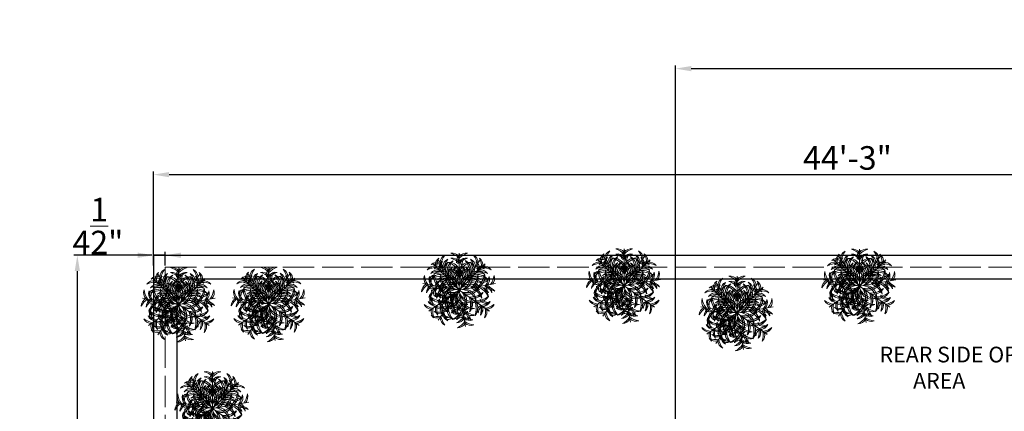
# Model space of a CAD drawing. Units: millimetres. Extents: x 595116 to 630915, y 909473 to 920225.
# Tile 124 of 134: x 629260 to 629637, y 920030 to 920179. Entities that reach past the tile are written whole.
import ezdxf

# ---------------------------------------------------------------- set-up
doc = ezdxf.new("R2010")
doc.units = ezdxf.units.MM
doc.linetypes.add('ACAD_ISO02W100', pattern=[15, 12, -3])
for name, color, linetype, lineweight in [('A-AREA-IDEN', 7, 'Continuous', 20), ('C-PROP', 7, 'Continuous', 25), ('C-PROP-REF', 240, 'ACAD_ISO02W100', 13), ('Dimension', 3, 'Continuous', 18), ('L-PLNT', 85, 'Continuous', 13)]:
    doc.layers.add(name, color=color, linetype=linetype, lineweight=lineweight)
doc.styles.get("Standard").update_dxf_attribs({"font": 'arial.ttf'})
doc.dimstyles.new('ISO-25', dxfattribs={"dimtxt": 9, "dimasz": 6, "dimexe": 1.25, "dimexo": 0.625, "dimtad": 1, "dimlunit": 4, "dimtxsty": 'Standard', "dimcen": 2.5, "dimadec": 0, "dimazin": 0, "dimtfac": 1, "dimtmove": 0, "dimatfit": 3, "dimfxl": 1, "dimarcsym": 0})

# ---------------------------------------------------------------- blocks, each defined once
blk = doc.blocks.new('A$C5D061C3B')
for p, q in [((3.377, 6.679), (3.377, 3.377)), ((1.03, 5.716), (3.365, 3.381)), ((1.483, 6.082), (3.377, 3.377)), ((5.259, 6.086), (3.365, 3.381)), ((5.712, 5.712), (3.377, 3.377)), ((0.125, 3.951), (3.377, 3.377)), ((6.629, 3.951), (3.377, 3.377)), ((0.66, 1.487), (3.365, 3.381)), ((1.483, 0.672), (3.377, 3.377)), ((6.07, 1.487), (3.365, 3.381)), ((3.951, 0.125), (3.377, 3.377)), ((6.082, 1.483), (3.377, 3.377))]:
    blk.add_line(p, q)
for centre, radius, start, end in [((1.998, 5.617), 0.762, 125.37567, 188.71003), ((3.066, 5.423), 1.715, 151.62064, 180.92372), ((2.419, 5.816), 0.762, 115.37567, 178.71003), ((3.438, 5.44), 1.715, 141.62064, 170.92372), ((2.763, 5.924), 0.762, 36.28997, 99.62433), ((2.145, 5.032), 1.715, 44.07628, 73.37936), ((2.763, 5.474), 0.762, 36.28997, 99.62433), ((2.145, 4.581), 1.715, 44.07628, 73.37936), ((3.901, 5.939), 0.762, 125.37567, 188.71003), ((4.969, 5.745), 1.715, 151.62064, 180.92372), ((3.991, 5.924), 0.762, 80.37567, 143.71003), ((4.61, 5.032), 1.715, 106.62064, 135.92372), ((3.991, 5.474), 0.762, 80.37567, 143.71003), ((4.61, 4.581), 1.715, 106.62064, 135.92372), ((3.871, 5.832), 0.38, 94.742, 213.74753), ((4.447, 5.681), 0.826, 139.61802, 183.21064), ((3.305, 5.444), 1.715, 9.07628, 38.37936), ((4.323, 5.82), 0.762, 1.28997, 64.62433), ((4.744, 5.613), 0.762, 351.28997, 54.62433), ((3.676, 5.419), 1.715, 359.07628, 28.37936), ((1.13, 4.748), 0.762, 81.28997, 144.62433), ((1.324, 3.68), 1.715, 89.07628, 118.37936), ((1.413, 5.111), 0.762, 71.28997, 134.62433), ((1.419, 4.026), 1.715, 79.07628, 108.37936), ((1.671, 4.742), 0.762, 71.28997, 134.62433), ((1.677, 3.657), 1.715, 79.07628, 108.37936), ((2.317, 5.298), 0.762, 125.37567, 188.71003), ((1.991, 5.462), 0.38, 139.742, 258.74753), ((3.385, 5.104), 1.715, 151.62064, 180.92372), ((2.505, 5.763), 0.826, 184.61802, 228.21064), ((2.678, 5.447), 0.762, 115.37567, 178.71003), ((3.035, 5.062), 1.056, 129.60629, 199.75109), ((3.696, 5.07), 1.715, 141.62064, 170.92372), ((3.894, 4.989), 1.77, 149.96343, 193.62881), ((3.344, 5.089), 1.056, 119.60629, 189.75109), ((2.422, 4.799), 1.056, 25.24891, 95.39371), ((1.866, 4.14), 1.77, 31.37119, 75.03657), ((3.46, 4.637), 1.056, 129.60629, 199.75109), ((4.177, 4.869), 1.77, 139.96343, 183.62881), ((4.319, 4.565), 1.77, 149.96343, 193.62881), ((3.688, 4.597), 1.056, 119.60629, 189.75109), ((4.522, 4.377), 1.77, 139.96343, 183.62881), ((4.332, 4.799), 1.056, 84.60629, 154.75109), ((4.888, 4.14), 1.77, 104.96343, 148.62881), ((2.221, 4.381), 1.77, 356.37119, 40.03657), ((3.054, 4.602), 1.056, 350.24891, 60.39371), ((3.398, 5.094), 1.056, 350.24891, 60.39371), ((2.565, 4.873), 1.77, 356.37119, 40.03657), ((3.283, 4.633), 1.056, 340.24891, 50.39371), ((2.424, 4.56), 1.77, 346.37119, 30.03657), ((2.848, 4.985), 1.77, 346.37119, 30.03657), ((3.707, 5.058), 1.056, 340.24891, 50.39371), ((4.064, 5.451), 0.762, 1.28997, 64.62433), ((3.046, 5.075), 1.715, 9.07628, 38.37936), ((5.065, 3.661), 1.715, 71.62064, 100.92372), ((5.071, 4.746), 0.762, 45.37567, 108.71003), ((3.357, 5.1), 1.715, 359.07628, 28.37936), ((4.425, 5.294), 0.762, 351.28997, 54.62433), ((5.564, 4.807), 0.762, 80.37567, 143.71003), ((6.182, 3.914), 1.715, 106.62064, 135.92372), ((5.419, 3.676), 1.715, 61.62064, 90.92372), ((5.613, 4.744), 0.762, 35.37567, 98.71003), ((0.975, 4.424), 0.762, 160.37567, 223.71003), ((1.962, 4.878), 1.715, 186.62064, 215.92372), ((1.419, 4.346), 0.762, 160.37567, 223.71003), ((2.405, 4.8), 1.715, 186.62064, 215.92372), ((1.12, 4.31), 0.38, 94.742, 213.74753), ((1.448, 4.43), 0.762, 81.28997, 144.62433), ((1.642, 3.362), 1.715, 89.07628, 118.37936), ((1.696, 4.159), 0.826, 139.61802, 183.21064), ((1.685, 3.712), 1.056, 70.24891, 140.39371), ((1.757, 2.853), 1.77, 76.37119, 120.03657), ((2.143, 4.564), 1.056, 164.60629, 234.75109), ((1.78, 3.994), 1.056, 60.24891, 130.39371), ((1.702, 3.136), 1.77, 66.37119, 110.03657), ((2.888, 4.998), 1.77, 184.96343, 228.62881), ((2.124, 3.502), 1.056, 60.24891, 130.39371), ((2.046, 2.644), 1.77, 66.37119, 110.03657), ((2.734, 4.46), 1.056, 164.60629, 234.75109), ((3.48, 4.893), 1.77, 184.96343, 228.62881), ((2.358, 3.686), 1.029, 3.42594, 103.63458), ((1.93, 3.14), 1.557, 21.66646, 83.18779), ((3.25, 4.435), 1.029, 156.36542, 256.57406), ((3.862, 4.761), 1.557, 176.81221, 238.33354), ((2.422, 4.198), 1.056, 25.24891, 95.39371), ((1.866, 3.54), 1.77, 31.37119, 75.03657), ((3.868, 4.321), 1.029, 121.36542, 221.57406), ((4.556, 4.237), 1.557, 141.81221, 203.33354), ((4.035, 4.215), 1.029, 111.36542, 211.57406), ((2.707, 4.219), 1.029, 328.42594, 68.63458), ((2.044, 4.017), 1.557, 346.66646, 48.18779), ((4.698, 4.013), 1.557, 131.81221, 193.33354), ((4.397, 3.686), 1.029, 76.36542, 176.57406), ((4.332, 4.198), 1.056, 84.60629, 154.75109), ((4.888, 3.54), 1.77, 104.96343, 148.62881), ((4.824, 3.14), 1.557, 96.81221, 158.33354), ((2.187, 4.233), 1.557, 336.66646, 38.18779), ((2.875, 4.316), 1.029, 318.42594, 58.63458), ((2.893, 4.761), 1.557, 301.66646, 3.18779), ((3.504, 4.435), 1.029, 283.42594, 23.63458), ((4.696, 2.648), 1.77, 69.96343, 113.62881), ((4.618, 3.506), 1.056, 49.60629, 119.75109), ((5.04, 3.14), 1.77, 69.96343, 113.62881), ((4.963, 3.998), 1.056, 49.60629, 119.75109), ((3.275, 4.893), 1.77, 311.37119, 355.03657), ((4.985, 2.848), 1.77, 59.96343, 103.62881), ((4.02, 4.46), 1.056, 305.24891, 15.39371), ((5.058, 3.707), 1.056, 39.60629, 109.75109), ((3.866, 4.998), 1.77, 311.37119, 355.03657), ((5.1, 3.357), 1.715, 61.62064, 90.92372), ((5.294, 4.425), 0.762, 35.37567, 98.71003), ((4.611, 4.564), 1.056, 305.24891, 15.39371), ((4.988, 5.812), 1.715, 279.07628, 308.37936), ((5.365, 4.794), 0.762, 271.28997, 334.62433), ((4.349, 4.8), 1.715, 324.07628, 353.37936), ((5.335, 4.346), 0.762, 316.28997, 19.62433), ((4.793, 4.878), 1.715, 324.07628, 353.37936), ((5.779, 4.424), 0.762, 316.28997, 19.62433), ((0.762, 3.214), 0.762, 116.28997, 179.62433), ((1.534, 2.451), 1.715, 124.07628, 153.37936), ((1.206, 3.136), 0.762, 116.28997, 179.62433), ((1.977, 2.373), 1.715, 124.07628, 153.37936), ((1.062, 4.452), 0.826, 229.61802, 273.21064), ((0.91, 3.875), 0.38, 184.742, 303.74753), ((1.811, 2.684), 1.056, 105.24891, 175.39371), ((2.363, 2.022), 1.77, 111.37119, 155.03657), ((2.185, 0.015), 3.567, 70.47721, 111.6585), ((1.588, 3.666), 0.38, 94.742, 213.74753), ((2.109, 3.287), 1.056, 70.24891, 140.39371), ((2.182, 2.428), 1.77, 76.37119, 120.03657), ((2.165, 3.515), 0.826, 139.61802, 183.21064), ((2.403, 2.58), 1.056, 105.24891, 175.39371), ((2.955, 1.917), 1.77, 111.37119, 155.03657), ((2.007, 3.071), 0.506, 93.87442, 233.97626), ((2.426, 2.879), 1.029, 48.42594, 148.63458), ((2.51, 2.191), 1.557, 66.66646, 128.18779), ((2.729, 4.702), 1.557, 221.81221, 283.33354), ((2.527, 4.039), 1.029, 201.36542, 301.57406), ((2.365, 3.045), 1.029, 38.42594, 138.63458), ((2.328, 2.353), 1.557, 56.66646, 118.18779), ((2.489, 2.932), 0.825, 128.75364, 199.09705), ((2.387, 3.752), 0.574, 99.98654, 199.40339), ((3.599, 3.314), 1.651, 142.57587, 170.89417), ((2.903, 2.8), 0.855, 116.44767, 194.36723), ((4.744, 1.779), 2.789, 140.40074, 163.13904), ((2.741, 3.253), 0.372, 114.22575, 255.12788), ((2.84, 3.739), 0.372, 69.22575, 210.12788), ((3.037, 3.338), 0.515, 150.43977, 228.66943), ((3.109, 3.59), 0.515, 105.43977, 183.66943), ((4.414, 2.358), 1.557, 61.81221, 123.33354), ((4.377, 3.05), 1.029, 41.36542, 141.57406), ((4.233, 2.187), 1.557, 51.81221, 113.33354), ((4.316, 2.875), 1.029, 31.36542, 131.57406), ((4.001, 4.702), 1.557, 256.66646, 318.18779), ((4.013, 4.698), 1.557, 256.66646, 318.18779), ((4.203, 4.039), 1.029, 238.42594, 338.63458), ((4.215, 4.035), 1.029, 238.42594, 338.63458), ((4.56, 2.424), 1.77, 59.96343, 103.62881), ((4.633, 3.283), 1.056, 39.60629, 109.75109), ((3.799, 1.917), 1.77, 24.96343, 68.62881), ((4.352, 2.58), 1.056, 4.60629, 74.75109), ((4.391, 2.022), 1.77, 24.96343, 68.62881), ((4.943, 2.684), 1.056, 4.60629, 74.75109), ((6.053, 3.533), 0.38, 146.25247, 265.258), ((4.777, 2.373), 1.715, 26.62064, 55.92372), ((6.629, 3.684), 0.826, 176.78936, 220.38198), ((5.935, 2.842), 0.762, 35.37567, 98.71003), ((5.549, 3.136), 0.762, 0.37567, 63.71003), ((1.067, 2.749), 0.376, 122.05775, 257.85325), ((1.873, 4.181), 1.77, 229.96343, 273.62881), ((1.653, 3.348), 1.056, 209.60629, 279.75109), ((1.122, 2.441), 0.38, 139.742, 258.74753), ((1.636, 2.741), 0.826, 184.61802, 228.21064), ((1.37, 2.745), 0.529, 140.18449, 223.65396), ((1.447, 3.129), 0.376, 122.05775, 257.85325), ((1.751, 3.126), 0.529, 140.18449, 223.65396), ((2.145, 3.693), 1.056, 209.60629, 279.75109), ((2.365, 4.526), 1.77, 229.96343, 273.62881), ((2.328, 4.401), 1.557, 241.81221, 303.33354), ((2.365, 3.709), 1.029, 221.36542, 321.57406), ((4.912, 0.157), 3.567, 115.47721, 156.6585), ((2.412, 2.943), 0.574, 144.98654, 244.40339), ((2.896, 2.427), 1.029, 83.42594, 183.63458), ((3.359, 1.911), 1.557, 101.66646, 163.18779), ((3.578, 3.49), 1.651, 187.57587, 215.89417), ((3.24, 2.128), 1.056, 150.24891, 220.39371), ((4.099, 2.051), 1.77, 156.37119, 200.03657), ((1.911, 3.359), 1.557, 286.81221, 348.33354), ((2.427, 2.896), 1.029, 266.36542, 6.57406), ((3.45, 2.634), 0.855, 161.44767, 239.36723), ((3.003, 2.844), 0.372, 159.22575, 300.12788), ((3.152, 3.113), 0.515, 195.43977, 273.66943), ((3.697, 2.369), 1.029, 128.42594, 228.63458), ((5.474, 3.214), 2.789, 185.40074, 208.13904), ((4.389, 2.332), 1.557, 146.66646, 208.18779), ((4.035, 2.539), 1.029, 148.42594, 248.63458), ((4.698, 2.741), 1.557, 166.66646, 228.18779), ((6.727, 2.189), 3.567, 160.47721, 201.6585), ((4.435, 3.25), 1.029, 193.42594, 293.63458), ((4.761, 3.862), 1.557, 211.66646, 273.18779), ((2.341, 2.332), 1.557, 331.81221, 33.33354), ((2.353, 2.328), 1.557, 331.81221, 33.33354), ((3.033, 2.369), 1.029, 311.36542, 51.57406), ((3.045, 2.365), 1.029, 311.36542, 51.57406), ((3.395, 1.911), 1.557, 16.81221, 78.33354), ((3.858, 2.427), 1.029, 356.36542, 96.57406), ((4.365, 4.526), 1.77, 266.37119, 310.03657), ((2.632, 2.051), 1.77, 339.96343, 23.62881), ((4.377, 4.522), 1.77, 266.37119, 310.03657), ((2.644, 2.046), 1.77, 339.96343, 23.62881), ((3.49, 2.128), 1.056, 319.60629, 29.75109), ((3.502, 2.124), 1.056, 319.60629, 29.75109), ((4.585, 3.693), 1.056, 260.24891, 330.39371), ((4.597, 3.688), 1.056, 260.24891, 330.39371), ((4.857, 4.181), 1.77, 266.37119, 310.03657), ((4.869, 4.177), 1.77, 266.37119, 310.03657), ((5.077, 3.348), 1.056, 260.24891, 330.39371), ((5.089, 3.344), 1.056, 260.24891, 330.39371), ((5.741, 1.774), 1.715, 61.62064, 90.92372), ((0.926, 2.424), 0.762, 205.37567, 268.71003), ((1.303, 3.442), 1.715, 231.62064, 260.92372), ((1.672, 3.7), 1.715, 231.62064, 260.92372), ((1.295, 2.682), 0.762, 205.37567, 268.71003), ((1.702, 3.619), 1.77, 249.96343, 293.62881), ((1.78, 2.76), 1.056, 229.60629, 299.75109), ((2, 1.676), 0.762, 161.28997, 224.62433), ((3.086, 1.681), 1.715, 169.07628, 198.37936), ((2.046, 4.111), 1.77, 249.96343, 293.62881), ((2.124, 3.252), 1.056, 229.60629, 299.75109), ((1.908, 2.317), 0.38, 139.742, 258.74753), ((2.422, 2.617), 0.826, 184.61802, 228.21064), ((2.748, 1.784), 1.056, 150.24891, 220.39371), ((2.188, 1.837), 0.376, 167.05775, 302.85325), ((3.607, 1.706), 1.77, 156.37119, 200.03657), ((2.405, 2.049), 0.529, 185.18449, 268.65396), ((2.624, 2.192), 0.506, 138.87442, 278.97626), ((3.064, 2.435), 0.825, 173.75364, 244.09705), ((3.344, 1.665), 1.056, 170.24891, 240.39371), ((4.177, 1.886), 1.77, 176.37119, 220.03657), ((3.428, 3.603), 1.651, 232.57587, 260.89417), ((2.99, 2.391), 0.574, 189.98654, 289.40339), ((3.688, 2.157), 1.056, 170.24891, 240.39371), ((1.917, 2.955), 1.77, 294.96343, 338.62881), ((2.58, 2.403), 1.056, 274.60629, 344.75109), ((4.522, 2.378), 1.77, 176.37119, 220.03657), ((3.81, 2.493), 0.825, 218.75364, 289.09705), ((3.671, 2.011), 0.506, 183.87442, 323.97626), ((3.942, 2.908), 0.855, 206.44767, 284.36723), ((4.963, 4.749), 2.789, 230.40074, 253.13904), ((4.893, 3.48), 1.77, 221.37119, 265.03657), ((4.46, 2.734), 1.056, 215.24891, 285.39371), ((3.124, 1.706), 1.77, 339.96343, 23.62881), ((3.136, 1.702), 1.77, 339.96343, 23.62881), ((3.982, 1.784), 1.056, 319.60629, 29.75109), ((3.994, 1.78), 1.056, 319.60629, 29.75109), ((5.385, 1.584), 0.38, 101.25247, 220.258), ((5.899, 1.283), 0.826, 131.78936, 175.38198), ((6.244, 3.948), 1.715, 234.07628, 263.37936), ((5.79, 2.962), 0.762, 226.28997, 289.62433), ((3.645, 1.681), 1.715, 341.62064, 10.92372), ((4.73, 1.676), 0.762, 315.37567, 18.71003), ((3.657, 1.677), 1.715, 341.62064, 10.92372), ((4.742, 1.671), 0.762, 315.37567, 18.71003), ((5.058, 3.7), 1.715, 279.07628, 308.37936), ((5.07, 3.696), 1.715, 279.07628, 308.37936), ((5.435, 2.682), 0.762, 271.28997, 334.62433), ((5.447, 2.678), 0.762, 271.28997, 334.62433), ((5.427, 3.442), 1.715, 279.07628, 308.37936), ((5.44, 3.438), 1.715, 279.07628, 308.37936), ((5.804, 2.424), 0.762, 271.28997, 334.62433), ((5.816, 2.419), 0.762, 271.28997, 334.62433), ((1.631, 1.417), 0.762, 161.28997, 224.62433), ((1.419, 2.729), 1.715, 251.62064, 280.92372), ((1.413, 1.643), 0.762, 225.37567, 288.71003), ((2.717, 1.423), 1.715, 169.07628, 198.37936), ((1.671, 2.012), 0.762, 225.37567, 288.71003), ((1.677, 3.098), 1.715, 251.62064, 280.92372), ((2.419, 0.938), 0.762, 181.28997, 244.62433), ((3.438, 1.315), 1.715, 189.07628, 218.37936), ((2.188, 1.299), 0.376, 167.05775, 302.85325), ((2.405, 1.511), 0.529, 185.18449, 268.65396), ((2.678, 1.307), 0.762, 181.28997, 244.62433), ((3.696, 1.684), 1.715, 189.07628, 218.37936), ((2.583, 1.701), 0.826, 229.61802, 273.21064), ((2.432, 1.124), 0.38, 184.742, 303.74753), ((3.227, 2.169), 0.826, 229.61802, 273.21064), ((3.076, 1.593), 0.38, 184.742, 303.74753), ((2.022, 2.363), 1.77, 294.96343, 338.62881), ((2.684, 1.811), 1.056, 274.60629, 344.75109), ((2.373, 1.977), 1.715, 296.62064, 325.92372), ((3.68, 0.113), 0.826, 86.78936, 130.38198), ((3.528, 0.69), 0.38, 56.25247, 175.258), ((3.616, 1.755), 0.529, 230.18449, 313.65396), ((3.613, 1.452), 0.376, 212.05775, 347.85325), ((3.997, 1.374), 0.529, 230.18449, 313.65396), ((4.998, 2.888), 1.77, 221.37119, 265.03657), ((3.994, 1.071), 0.376, 212.05775, 347.85325), ((4.564, 2.143), 1.056, 215.24891, 285.39371), ((4.8, 2.405), 1.715, 234.07628, 263.37936), ((4.79, 1.377), 0.762, 181.28997, 244.62433), ((5.808, 1.754), 1.715, 189.07628, 218.37936), ((4.014, 1.423), 1.715, 341.62064, 10.92372), ((5.099, 1.417), 0.762, 315.37567, 18.71003), ((3.136, 1.206), 0.762, 270.37567, 333.71003), ((2.451, 1.534), 1.715, 296.62064, 325.92372), ((3.214, 0.762), 0.762, 270.37567, 333.71003), ((4.346, 1.419), 0.762, 226.28997, 289.62433), ((4.878, 1.962), 1.715, 234.07628, 263.37936), ((4.424, 0.975), 0.762, 226.28997, 289.62433)]:
    blk.add_arc(centre, radius, start, end)
blk = doc.blocks.new('*D125')
at = {"layer": 'Defpoints', "color": 0, "transparency": 16777216}
for p in [(629842.54, 920120.25), (629311.54, 920089.43), (629842.54, 920089.43)]:
    blk.add_point(p, dxfattribs=at)
at = {"layer": 'Dimension', "color": 0, "lineweight": -2, "transparency": 16777216}
for p, q in [((629311.54, 920090.05), (629311.54, 920121.5)), ((629317.54, 920120.25), (629836.54, 920120.25)), ((629842.54, 920090.05), (629842.54, 920121.5))]:
    blk.add_line(p, q, dxfattribs=at)
at = {"layer": 'Dimension', "color": 0, "transparency": 16777216}
for points in [[(629317.54, 920121.25), (629317.54, 920119.25), (629311.54, 920120.25)], [(629836.54, 920121.25), (629836.54, 920119.25), (629842.54, 920120.25)]]:
    blk.add_solid(points, dxfattribs=at)
at = {"layer": 'Dimension', "color": 0, "transparency": 16777216, "insert": (629577.04, 920125.47), "char_height": 9, "attachment_point": 5}
blk.add_mtext('44\'-3"', dxfattribs=at)
blk = doc.blocks.new('*D127')
at = {"layer": 'Defpoints', "color": 0, "transparency": 16777216}
for p in [(629311.54, 920089.45), (629311.54, 920084.93), (629316.04, 920084.93)]:
    blk.add_point(p, dxfattribs=at)
at = {"layer": 'Dimension', "color": 0, "lineweight": -2, "transparency": 16777216}
for p, q in [((629305.54, 920089.45), (629281.02, 920089.45)), ((629311.54, 920085.55), (629311.54, 920090.7)), ((629316.04, 920089.45), (629311.54, 920089.45)), ((629316.04, 920085.55), (629316.04, 920090.7)), ((629322.04, 920089.45), (629328.04, 920089.45))]:
    blk.add_line(p, q, dxfattribs=at)
at = {"layer": 'Dimension', "color": 0, "transparency": 16777216}
for points in [[(629305.54, 920090.45), (629305.54, 920088.45), (629311.54, 920089.45)], [(629322.04, 920090.45), (629322.04, 920088.45), (629316.04, 920089.45)]]:
    blk.add_solid(points, dxfattribs=at)
at = {"layer": 'Dimension', "color": 0, "transparency": 16777216, "insert": (629290.28, 920100.61), "char_height": 9, "attachment_point": 5}
blk.add_mtext('4{\\H1x;\\S1/2;}"', dxfattribs=at)
blk = doc.blocks.new('*D128')
at = {"layer": 'Defpoints', "color": 0, "transparency": 16777216}
for p in [(629311.54, 920089.43), (629282.4, 919141.93), (629311.54, 919141.93)]:
    blk.add_point(p, dxfattribs=at)
at = {"layer": 'Dimension', "color": 0, "lineweight": -2, "transparency": 16777216}
for p, q in [((629310.92, 920089.43), (629281.15, 920089.43)), ((629282.4, 920083.43), (629282.4, 919147.93)), ((629310.92, 919141.93), (629281.15, 919141.93))]:
    blk.add_line(p, q, dxfattribs=at)
at = {"layer": 'Dimension', "color": 0, "transparency": 16777216}
for points in [[(629281.4, 920083.43), (629283.4, 920083.43), (629282.4, 920089.43)], [(629281.4, 919147.93), (629283.4, 919147.93), (629282.4, 919141.93)]]:
    blk.add_solid(points, dxfattribs=at)
at = {"layer": 'Dimension', "color": 0, "transparency": 16777216, "insert": (629271.16, 919615.68), "char_height": 9, "attachment_point": 5, "rotation": 90}
blk.add_mtext('78\'-11{\\H1x;\\S1/2;}"', dxfattribs=at)
blk = doc.blocks.new('*D220')
at = {"layer": 'Defpoints', "color": 0, "transparency": 16777216}
for p in [(629824.95, 920160.76), (629511.27, 919302.01), (629824.95, 919302.01)]:
    blk.add_point(p, dxfattribs=at)
at = {"layer": 'Dimension', "color": 0, "lineweight": -2, "transparency": 16777216}
for p, q in [((629511.27, 919302.63), (629511.27, 920162.01)), ((629517.27, 920160.76), (629818.95, 920160.76)), ((629824.95, 919302.63), (629824.95, 920162.01))]:
    blk.add_line(p, q, dxfattribs=at)
at = {"layer": 'Dimension', "color": 0, "transparency": 16777216}
for points in [[(629517.27, 920161.76), (629517.27, 920159.76), (629511.27, 920160.76)], [(629818.95, 920161.76), (629818.95, 920159.76), (629824.95, 920160.76)]]:
    blk.add_solid(points, dxfattribs=at)
at = {"layer": 'Dimension', "color": 0, "transparency": 16777216, "insert": (629668.11, 920166.03), "char_height": 9, "attachment_point": 5}
blk.add_mtext('26\'-1 1/2"', dxfattribs=at)

msp = doc.modelspace()

# ---------------------------------------------------------------- linework, layer by layer
at = {"layer": 'C-PROP'}
for p, q in [((629311.541, 920089.428), (629311.541, 919957.928)), ((629320.541, 920080.428), (629833.541, 920080.428)), ((629320.541, 919957.928), (629320.541, 920080.428))]:
    msp.add_line(p, q, dxfattribs=at)
msp.add_lwpolyline([(629311.541, 920089.428), (629842.541, 920089.428)], dxfattribs=at)
at = {"layer": 'C-PROP-REF'}
for p, q in [((629316.041, 920084.928), (629838.041, 920084.928)), ((629316.041, 919146.428), (629316.041, 920084.928))]:
    msp.add_line(p, q, dxfattribs=at)

# ---------------------------------------------------------------- block references
at = {"layer": 'L-PLNT', "xscale": 4.271269117679152, "yscale": 4.271269117679152, "zscale": 4.271269117679152}
for p in [(629414.08, 920061.719), (629477.177, 920063.335), (629567.274, 920063.243), (629306.856, 920056.216), (629341.275, 920056.33), (629520.357, 920052.884), (629319.703, 920016.452)]:
    msp.add_blockref('A$C5D061C3B', p, dxfattribs=at)

# ---------------------------------------------------------------- texts
at = {"layer": 'A-AREA-IDEN', "insert": (629589.324, 920054.511), "char_height": 6, "attachment_point": 1}
msp.add_mtext_dynamic_manual_height_columns('{REAR SIDE OPEN\\P       AREA}', width=127.44285, gutter_width=12.5, heights=[0], dxfattribs=at)

# ---------------------------------------------------------------- dimensions: what is measured, and where the dimension line sits
at = {"layer": 'Dimension'}
for base, p1, p2, override, picture, middle in [((629824.951, 920160.756), (629511.274, 919302.009), (629824.951, 919302.009), {"dimdec": 1, "dimlfac": 1, "dimrnd": 0, "dimzin": 1, "dimdsep": 46, "dimlunit": 4, "dimfrac": 2}, '*D220', (629668.113, 920166.035)), ((629842.541, 920120.249), (629311.541, 920089.428), (629842.541, 920089.428), {"dimclrd": 0, "dimclre": 0, "dimclrt": 0}, '*D125', (629577.041, 920125.472)), ((629311.541, 920089.453), (629316.041, 920084.928), (629311.541, 920084.928), {"dimclrd": 0, "dimclre": 0, "dimclrt": 0}, '*D127', (629290.281, 920100.614))]:
    dim = msp.add_linear_dim(base=base, p1=p1, p2=p2, dimstyle='ISO-25', override=override, dxfattribs=at)
    dim.commit()
    dim.dimension.update_dxf_attribs({"geometry": picture, "text_midpoint": middle})
dim = msp.add_linear_dim(base=(629282.395, 919141.928), p1=(629311.541, 920089.428), p2=(629311.541, 919141.928), angle=90, dimstyle='ISO-25', override={"dimclrd": 0, "dimclre": 0, "dimclrt": 0}, dxfattribs=at)
dim.commit()
dim.dimension.update_dxf_attribs({"geometry": '*D128', "text_midpoint": (629271.157, 919615.678)})

doc.saveas('drawing.dxf')
